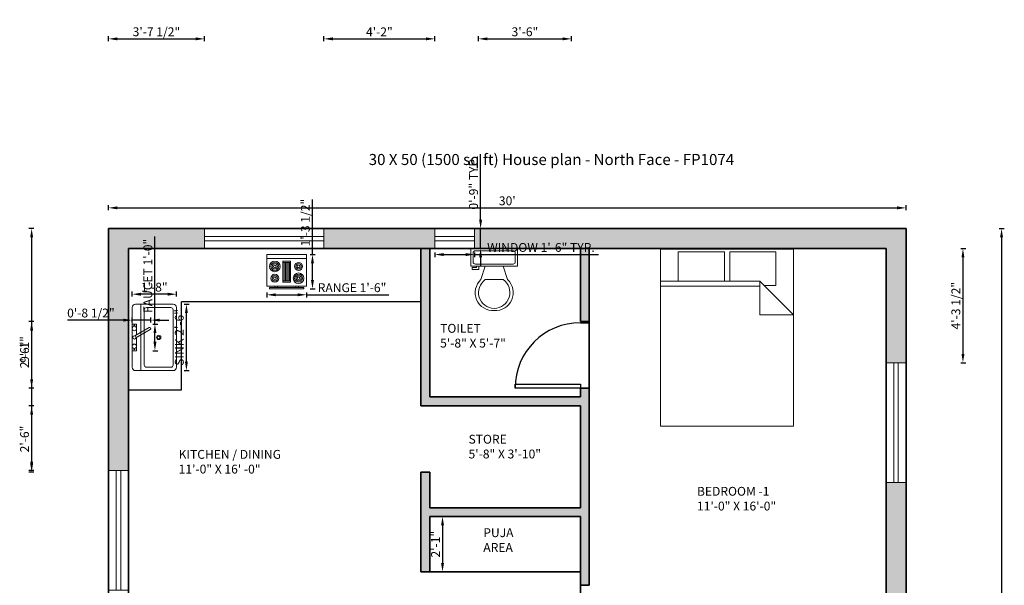
# Model space of a CAD drawing. Units: inches. Extents: x -40 to 407, y -627 to 108.
# Tile 2 of 2: x -37 to 407, y -147 to 108. Entities that reach past the tile are written whole.
import ezdxf

# ---------------------------------------------------------------- set-up
doc = ezdxf.new("R2010")
doc.units = ezdxf.units.IN
for name, color, linetype, lineweight in [('A-ANNO-DIMS', 2, 'Continuous', 18), ('A-ANNO-TEXT', 7, 'Continuous', 18), ('A-AREA-IDEN', 7, 'Continuous', 18), ('A-DOOR', 4, 'Continuous', 25), ('A-EQPM', 9, 'Continuous', 18), ('A-FLOR-CASE', 7, 'Continuous', 25), ('A-FLOR-FIXT', 8, 'Continuous', 18), ('A-FURN', 8, 'Continuous', 18), ('A-GLAZ', 6, 'Continuous', 18), ('A-WALL', 7, 'Continuous', 35), ('A-WALL-PATT', 251, 'Continuous', 13)]:
    doc.layers.add(name, color=color, linetype=linetype, lineweight=lineweight)
doc.styles.get("Standard").update_dxf_attribs({"font": 'arial.ttf'})
doc.dimstyles.new('ISO-25', dxfattribs={"dimtxt": 4, "dimasz": 4, "dimexe": 1.25, "dimexo": 0.625, "dimtad": 1, "dimlunit": 3, "dimtxsty": 'Standard', "dimcen": 2.5, "dimadec": 0, "dimazin": 0, "dimtfac": 1, "dimtmove": 0, "dimatfit": 3, "dimfxl": 1, "dimfxlon": 1, "dimarcsym": 0})

# ---------------------------------------------------------------- blocks, each defined once
blk = doc.blocks.new('*U4')
for p, q in [((0, 0), (0, -100)), ((750, 0), (750, -100))]:
    blk.add_line(p, q)
blk.add_lwpolyline([(0, 0), (0, 750), (43.75, 750), (43.75, 0)], close=True)
blk.add_arc((0, 0), 750, 0, 90)
blk = doc.blocks.new('*U2')
for p, q in [((9.5, -6), (9.5, -2)), ((-10, -8.5), (-8, -8.5)), ((-10, -9.5), (-10, -8.5)), ((-8, -8.5), (-8, -8)), ((-7, -8), (-7, -9.5)), ((-4, -8), (-6, -14)), ((4, -8), (6, -14)), ((-7, -9.5), (-10, -9.5)), ((4, -14), (-4, -14))]:
    blk.add_line(p, q)
blk.add_lwpolyline([(10.5, -8), (10.5, 0), (-10.5, 0), (-10.5, -8)], close=True)
for points in [[(-9.5, -2), (-9.5, -6)], [(8.5, -1), (-8.5, -1)], [(-8.5, -7), (8.5, -7)]]:
    blk.add_lwpolyline(points)
for centre, radius, start, end in [((-8.625, -1.875), 0.8839, 81.8699, 188.1301), ((8.625, -1.875), 0.8839, 351.8699, 98.1301), ((-8.625, -6.125), 0.8839, 171.869898, 278.1301), ((8.625, -6.125), 0.8839, 261.8699, 8.1301), ((-0.4772, -19.9188), 8.0953, 133.01722, 273.38), ((0.0374, -19.8731), 7.127, 124.50543, 269.7), ((-0.0373, -19.8731), 7.127, 270.3, 55.4946), ((0.4773, -19.9188), 8.0953, 266.62, 46.9828)]:
    blk.add_arc(centre, radius, start, end)
blk = doc.blocks.new('Sink-single - 30 in top')
blk.add_line((-15, -3.999996), (15, -3.999996))
for points in [[(-13.5, 0), (13.5, 0)], [(-15, -18.499996), (-15, -1.5)], [(15, -1.5), (15, -18.499996)], [(-13.5, -17.499996), (-13.5, -6.499996)], [(-12.5, -5.499996), (12.5, -5.499996)], [(13.5, -6.499996), (13.5, -17.499996)], [(13.5, -19.999996), (-13.5, -19.999996)], [(12.5, -18.499996), (-12.5, -18.499996)]]:
    blk.add_lwpolyline(points)
for radius in [1, 0.5]:
    blk.add_circle((0, -11.999996), radius)
for centre, radius, start, end in [((-13.5, -1.5), 1.5, 90, 180), ((13.5, -1.5), 1.5, 0, 90), ((-12.5, -6.499996), 1, 90, 180), ((12.5, -6.499996), 1, 0, 90), ((-12.5, -17.499996), 1, 180, 270), ((12.5, -17.499996), 1, 270, 0), ((-13.5, -18.499996), 1.5, 180, 270), ((13.5, -18.499996), 1.5, 270, 0)]:
    blk.add_arc(centre, radius, start, end)
blk = doc.blocks.new('Faucet - kit sink top')
for p, q in [((-5.5, -0.75), (-5.5, -1.25)), ((-4.94278, -0.75), (-5.5, -0.75)), ((-5.5, -1.25), (-4.94278, -1.25)), ((-0.14775, -1.7441), (3.56698, -8.1782)), ((4.43301, -7.6782), (0.71828, -1.2441)), ((4.94278, -0.75), (5.5, -0.75)), ((5.5, -1.25), (4.94278, -1.25)), ((5.5, -0.75), (5.5, -1.25))]:
    blk.add_line(p, q)
blk.add_lwpolyline([(-0.00587, -2), (-6, -2), (-6, 0), (6, 0), (6, -2), (1.15195, -2)])
for centre, radius in [((-4, -1), 1), ((4, -1), 1), ((0, -1), 0.75)]:
    blk.add_circle(centre, radius)
blk.add_arc((4, -7.9282), 0.5, 210, 30)
blk = doc.blocks.new('Range-Oven - 30 in top')
for p, q in [((0, -3), (30, -3)), ((12, -6), (18, -6)), ((13, -20), (13, -6)), ((14, -6), (14, -20)), ((15, -20), (15, -6)), ((16, -6), (16, -20)), ((17, -20), (17, -6)), ((18, -20), (12, -20)), ((6, -24), (6, -25)), ((8, -25), (8, -24)), ((22, -25), (22, -24)), ((24, -24), (24, -25))]:
    blk.add_line(p, q)
for points in [[(0, -24), (0, 0), (30, 0), (30, -24)], [(12, -21), (12, -5), (18, -5), (18, -21)], [(2, -26), (2, -25), (28, -25), (28, -26)]]:
    blk.add_lwpolyline(points, close=True)
for centre, radius in [((6, -9), 4), ((6, -9), 3), ((6, -9), 2), ((24, -9), 3), ((24, -9), 2), ((6, -9), 1), ((24, -18), 4), ((24, -9), 1), ((6, -18), 3), ((6, -18), 2), ((6, -18), 1), ((24, -18), 3), ((24, -18), 2), ((24, -18), 1)]:
    blk.add_circle(centre, radius)
blk = doc.blocks.new('Bed - Queen')
for p, q in [((0, -80.00003), (0, 0)), ((0, 0), (59.99999, 0)), ((59.99999, 0), (59.99999, -80.00003)), ((7.99999, -1.2), (28.79998, -1.2)), ((7.99999, -14.4), (7.99999, -1.2)), ((28.79998, -1.2), (28.79998, -14.4)), ((31.19999, -1.2), (51.99999, -1.2)), ((31.19999, -14.4), (31.19999, -1.2)), ((51.99999, -1.2), (51.99999, -16.4)), ((0, -14.4), (44.8, -14.4)), ((44.8, -16.8), (0, -16.8)), ((59.99999, -29.6), (44.8, -14.4)), ((44.8, -14.4), (44.8, -29.6)), ((51.99999, -16.4), (46.79936, -16.4)), ((44.8, -29.6), (59.99999, -29.6)), ((59.99999, -80.00003), (0, -80.00003))]:
    blk.add_line(p, q)
blk = doc.blocks.new('*D9')
at = {"layer": 'A-ANNO-DIMS', "color": 0, "lineweight": -2, "transparency": 16777216}
for p, q in [((152.9, -116.12), (155.15, -116.12)), ((153.9, -120.12), (153.9, -137.12)), ((152.9, -141.12), (155.15, -141.12))]:
    blk.add_line(p, q, dxfattribs=at)
at = {"layer": 'A-ANNO-DIMS', "color": 0, "transparency": 16777216}
for points in [[(153.23, -120.12), (154.56, -120.12), (153.9, -116.12)], [(153.23, -137.12), (154.56, -137.12), (153.9, -141.12)]]:
    blk.add_solid(points, dxfattribs=at)
at = {"layer": 'Defpoints', "color": 0, "transparency": 16777216}
for p in [(148.12, -116.12), (148.12, -141.12), (153.9, -141.12)]:
    blk.add_point(p, dxfattribs=at)
at = {"layer": 'A-ANNO-DIMS', "color": 0, "transparency": 16777216, "insert": (151.26, -128.62), "char_height": 4, "attachment_point": 5, "rotation": 90}
blk.add_mtext('2\'-1"', dxfattribs=at)
blk = doc.blocks.new('*D13')
at = {"layer": 'A-ANNO-DIMS', "color": 0, "lineweight": -2, "transparency": 16777216}
for p, q in [((3.12, 22.26), (3.12, 24.51)), ((7.12, 23.26), (359.12, 23.26)), ((363.12, 22.26), (363.12, 24.51))]:
    blk.add_line(p, q, dxfattribs=at)
at = {"layer": 'A-ANNO-DIMS', "color": 0, "transparency": 16777216}
for points in [[(7.12, 23.93), (7.12, 22.59), (3.12, 23.26)], [(359.12, 23.93), (359.12, 22.59), (363.12, 23.26)]]:
    blk.add_solid(points, dxfattribs=at)
at = {"layer": 'Defpoints', "color": 0, "transparency": 16777216}
for p in [(363.12, 23.26), (3.12, 13.88), (363.12, 13.88)]:
    blk.add_point(p, dxfattribs=at)
at = {"layer": 'A-ANNO-DIMS', "color": 0, "transparency": 16777216, "insert": (183.12, 25.93), "char_height": 4, "attachment_point": 5}
blk.add_mtext("30'", dxfattribs=at)
blk = doc.blocks.new('*D14')
at = {"layer": 'A-ANNO-DIMS', "color": 0, "lineweight": -2, "transparency": 16777216}
for p, q in [((405.24, 13.88), (407.49, 13.88)), ((406.24, 9.88), (406.24, -582.12)), ((405.24, -586.12), (407.49, -586.12))]:
    blk.add_line(p, q, dxfattribs=at)
at = {"layer": 'A-ANNO-DIMS', "color": 0, "transparency": 16777216}
for points in [[(405.57, 9.88), (406.91, 9.88), (406.24, 13.88)], [(405.57, -582.12), (406.91, -582.12), (406.24, -586.12)]]:
    blk.add_solid(points, dxfattribs=at)
at = {"layer": 'Defpoints', "color": 0, "transparency": 16777216}
for p in [(363.12, 13.88), (363.12, -586.12), (406.24, -586.12)]:
    blk.add_point(p, dxfattribs=at)
at = {"layer": 'A-ANNO-DIMS', "color": 0, "transparency": 16777216, "insert": (403.57, -286.12), "char_height": 4, "attachment_point": 5, "rotation": 90}
blk.add_mtext("50'", dxfattribs=at)
blk = doc.blocks.new('WIN-54IN')
for p, q in [((3.5, 54), (3.5, 0)), ((5.5, 54), (5.5, 0))]:
    blk.add_line(p, q)
blk.add_lwpolyline([(0, 54), (9, 54), (9, 0), (0, 0)], close=True)
blk = doc.blocks.new('WIN-18IN')
for p, q in [((18, 5.5), (0, 5.5)), ((18, 3.5), (0, 3.5))]:
    blk.add_line(p, q)
blk.add_lwpolyline([(0, 9), (18, 9), (18, 0), (0, 0)], close=True)
blk = doc.blocks.new('*D21')
at = {"layer": 'A-ANNO-DIMS', "color": 0, "lineweight": -2, "transparency": 16777216}
for p, q in [((150.38, 3.18), (150.38, 0.93)), ((154.38, 2.18), (164.38, 2.18)), ((168.38, 3.18), (168.38, 0.93)), ((168.38, 2.18), (224.25, 2.18))]:
    blk.add_line(p, q, dxfattribs=at)
at = {"layer": 'A-ANNO-DIMS', "color": 0, "transparency": 16777216}
for points in [[(154.38, 2.85), (154.38, 1.51), (150.38, 2.18)], [(164.38, 2.85), (164.38, 1.51), (168.38, 2.18)]]:
    blk.add_solid(points, dxfattribs=at)
at = {"layer": 'Defpoints', "color": 0, "transparency": 16777216}
for p in [(150.38, 4.88), (168.38, 4.88), (168.38, 2.18)]:
    blk.add_point(p, dxfattribs=at)
at = {"layer": 'A-ANNO-DIMS', "color": 0, "transparency": 16777216, "insert": (198.31, 4.87), "char_height": 4, "attachment_point": 5}
blk.add_mtext('WINDOW 1\'-6" TYP.', dxfattribs=at)
blk = doc.blocks.new('*D22')
at = {"layer": 'A-ANNO-DIMS', "color": 0, "lineweight": -2, "transparency": 16777216}
for p, q in [((171.08, 17.88), (171.08, 47.51)), ((170.08, 13.88), (172.33, 13.88)), ((171.08, 4.88), (171.08, 13.88)), ((170.08, 4.88), (172.33, 4.88)), ((171.08, 0.88), (171.08, -3.12))]:
    blk.add_line(p, q, dxfattribs=at)
at = {"layer": 'A-ANNO-DIMS', "color": 0, "transparency": 16777216}
for points in [[(170.41, 17.88), (171.75, 17.88), (171.08, 13.88)], [(170.41, 0.88), (171.75, 0.88), (171.08, 4.88)]]:
    blk.add_solid(points, dxfattribs=at)
at = {"layer": 'Defpoints', "color": 0, "transparency": 16777216}
for p in [(168.38, 13.88), (171.08, 13.88), (168.38, 4.88)]:
    blk.add_point(p, dxfattribs=at)
at = {"layer": 'A-ANNO-DIMS', "color": 0, "transparency": 16777216, "insert": (168.41, 34.7), "char_height": 4, "attachment_point": 5, "rotation": 90}
blk.add_mtext('0\'-9" TYP.', dxfattribs=at)
blk = doc.blocks.new('*D23')
at = {"layer": 'A-ANNO-DIMS', "color": 0, "lineweight": -2, "transparency": 16777216}
for p, q in [((37.28, -20.23), (39.53, -20.23)), ((38.28, -46.23), (38.28, -24.23)), ((37.28, -50.23), (39.53, -50.23))]:
    blk.add_line(p, q, dxfattribs=at)
at = {"layer": 'A-ANNO-DIMS', "color": 0, "transparency": 16777216}
for points in [[(37.62, -24.23), (38.95, -24.23), (38.28, -20.23)], [(37.62, -46.23), (38.95, -46.23), (38.28, -50.23)]]:
    blk.add_solid(points, dxfattribs=at)
at = {"layer": 'Defpoints', "color": 0, "transparency": 16777216}
for p in [(33.78, -20.23), (38.28, -20.23), (33.78, -50.23)]:
    blk.add_point(p, dxfattribs=at)
at = {"layer": 'A-ANNO-DIMS', "color": 0, "transparency": 16777216, "insert": (35.59, -35.23), "char_height": 4, "attachment_point": 5, "rotation": 90}
blk.add_mtext('SINK 2\'-6"', dxfattribs=at)
blk = doc.blocks.new('*D24')
at = {"layer": 'A-ANNO-DIMS', "color": 0, "lineweight": -2, "transparency": 16777216}
for p, q in [((13.78, -16.73), (13.78, -14.48)), ((29.78, -15.73), (17.78, -15.73)), ((33.78, -16.73), (33.78, -14.48))]:
    blk.add_line(p, q, dxfattribs=at)
at = {"layer": 'A-ANNO-DIMS', "color": 0, "transparency": 16777216}
for points in [[(17.78, -15.06), (17.78, -16.4), (13.78, -15.73)], [(29.78, -15.06), (29.78, -16.4), (33.78, -15.73)]]:
    blk.add_solid(points, dxfattribs=at)
at = {"layer": 'Defpoints', "color": 0, "transparency": 16777216}
for p in [(13.78, -15.73), (13.78, -20.23), (33.78, -20.23)]:
    blk.add_point(p, dxfattribs=at)
at = {"layer": 'A-ANNO-DIMS', "color": 0, "transparency": 16777216, "insert": (23.78, -13.06), "char_height": 4, "attachment_point": 5}
blk.add_mtext('1\'-8"', dxfattribs=at)
blk = doc.blocks.new('*D25')
at = {"layer": 'A-ANNO-DIMS', "color": 0, "lineweight": -2, "transparency": 16777216}
for p, q in [((24.08, -29.23), (24.08, 10.33)), ((23.08, -29.23), (25.33, -29.23)), ((24.08, -37.23), (24.08, -33.23)), ((23.08, -41.23), (25.33, -41.23))]:
    blk.add_line(p, q, dxfattribs=at)
at = {"layer": 'A-ANNO-DIMS', "color": 0, "transparency": 16777216}
for points in [[(23.42, -33.23), (24.75, -33.23), (24.08, -29.23)], [(23.42, -37.23), (24.75, -37.23), (24.08, -41.23)]]:
    blk.add_solid(points, dxfattribs=at)
at = {"layer": 'Defpoints', "color": 0, "transparency": 16777216}
for p in [(22.28, -29.23), (24.08, -29.23), (22.28, -41.23)]:
    blk.add_point(p, dxfattribs=at)
at = {"layer": 'A-ANNO-DIMS', "color": 0, "transparency": 16777216, "insert": (21.39, -7.45), "char_height": 4, "attachment_point": 5, "rotation": 90}
blk.add_mtext('FAUCET 1\'-0"', dxfattribs=at)
blk = doc.blocks.new('*D26')
at = {"layer": 'A-ANNO-DIMS', "color": 0, "lineweight": -2, "transparency": 16777216}
for p, q in [((13.78, -28.43), (13.78, -26.18)), ((22.28, -28.43), (22.28, -26.18)), ((9.78, -27.43), (-15.42, -27.43)), ((22.28, -27.43), (13.78, -27.43)), ((26.28, -27.43), (30.28, -27.43))]:
    blk.add_line(p, q, dxfattribs=at)
at = {"layer": 'A-ANNO-DIMS', "color": 0, "transparency": 16777216}
for points in [[(9.78, -26.76), (9.78, -28.1), (13.78, -27.43)], [(26.28, -26.76), (26.28, -28.1), (22.28, -27.43)]]:
    blk.add_solid(points, dxfattribs=at)
at = {"layer": 'Defpoints', "color": 0, "transparency": 16777216}
for p in [(13.78, -27.43), (13.78, -29.23), (22.28, -29.23)]:
    blk.add_point(p, dxfattribs=at)
at = {"layer": 'A-ANNO-DIMS', "color": 0, "transparency": 16777216, "insert": (-4.82, -24.74), "char_height": 4, "attachment_point": 5}
blk.add_mtext('0\'-8 1/2"', dxfattribs=at)
blk = doc.blocks.new('*D27')
at = {"layer": 'A-ANNO-DIMS', "color": 0, "lineweight": -2, "transparency": 16777216}
for p, q in [((74.61, -14.99), (74.61, -17.24)), ((78.61, -15.99), (88.5, -15.99)), ((92.5, -14.99), (92.5, -17.24)), ((92.5, -15.99), (129.6, -15.99))]:
    blk.add_line(p, q, dxfattribs=at)
at = {"layer": 'A-ANNO-DIMS', "color": 0, "transparency": 16777216}
for points in [[(78.61, -15.32), (78.61, -16.66), (74.61, -15.99)], [(88.5, -15.32), (88.5, -16.66), (92.5, -15.99)]]:
    blk.add_solid(points, dxfattribs=at)
at = {"layer": 'Defpoints', "color": 0, "transparency": 16777216}
for p in [(74.61, -13.31), (92.5, -13.31), (92.5, -15.99)]:
    blk.add_point(p, dxfattribs=at)
at = {"layer": 'A-ANNO-DIMS', "color": 0, "transparency": 16777216, "insert": (113.05, -13.3), "char_height": 4, "attachment_point": 5}
blk.add_mtext('RANGE 1\'-6"', dxfattribs=at)
blk = doc.blocks.new('*D28')
at = {"layer": 'A-ANNO-DIMS', "color": 0, "lineweight": -2, "transparency": 16777216}
for p, q in [((95.18, 2.2), (95.18, 27.02)), ((94.18, 2.2), (96.43, 2.2)), ((95.18, -9.31), (95.18, -1.8)), ((94.18, -13.31), (96.43, -13.31))]:
    blk.add_line(p, q, dxfattribs=at)
at = {"layer": 'A-ANNO-DIMS', "color": 0, "transparency": 16777216}
for points in [[(94.52, -1.8), (95.85, -1.8), (95.18, 2.2)], [(94.52, -9.31), (95.85, -9.31), (95.18, -13.31)]]:
    blk.add_solid(points, dxfattribs=at)
at = {"layer": 'Defpoints', "color": 0, "transparency": 16777216}
for p in [(92.5, 2.2), (95.18, 2.2), (92.5, -13.31)]:
    blk.add_point(p, dxfattribs=at)
at = {"layer": 'A-ANNO-DIMS', "color": 0, "transparency": 16777216, "insert": (92.49, 16.61), "char_height": 4, "attachment_point": 5, "rotation": 90}
blk.add_mtext('1\'-3 1/2"', dxfattribs=at)
blk = doc.blocks.new('*D29')
at = {"layer": 'A-ANNO-DIMS', "color": 0, "lineweight": -2, "transparency": 16777216}
for p, q in [((3.12, 98.58), (3.12, 100.83)), ((7.12, 99.58), (42.39, 99.58)), ((46.39, 98.58), (46.39, 100.83))]:
    blk.add_line(p, q, dxfattribs=at)
at = {"layer": 'A-ANNO-DIMS', "color": 0, "transparency": 16777216}
for points in [[(7.12, 100.25), (7.12, 98.91), (3.12, 99.58)], [(42.39, 100.25), (42.39, 98.91), (46.39, 99.58)]]:
    blk.add_solid(points, dxfattribs=at)
at = {"layer": 'Defpoints', "color": 0, "transparency": 16777216}
for p in [(46.39, 99.58), (3.12, 13.88), (46.39, 13.88)]:
    blk.add_point(p, dxfattribs=at)
at = {"layer": 'A-ANNO-DIMS', "color": 0, "transparency": 16777216, "insert": (24.75, 102.27), "char_height": 4, "attachment_point": 5}
blk.add_mtext('3\'-7 1/2"', dxfattribs=at)
blk = doc.blocks.new('*D30')
at = {"layer": 'A-ANNO-DIMS', "color": 0, "lineweight": -2, "transparency": 16777216}
for p, q in [((100.39, 98.58), (100.39, 100.83)), ((104.39, 99.58), (146.38, 99.58)), ((150.38, 98.58), (150.38, 100.83))]:
    blk.add_line(p, q, dxfattribs=at)
at = {"layer": 'A-ANNO-DIMS', "color": 0, "transparency": 16777216}
for points in [[(104.39, 100.25), (104.39, 98.91), (100.39, 99.58)], [(146.38, 100.25), (146.38, 98.91), (150.38, 99.58)]]:
    blk.add_solid(points, dxfattribs=at)
at = {"layer": 'Defpoints', "color": 0, "transparency": 16777216}
for p in [(150.38, 99.58), (100.39, 13.88), (150.38, 13.88)]:
    blk.add_point(p, dxfattribs=at)
at = {"layer": 'A-ANNO-DIMS', "color": 0, "transparency": 16777216, "insert": (125.39, 102.21), "char_height": 4, "attachment_point": 5}
blk.add_mtext('4\'-2"', dxfattribs=at)
blk = doc.blocks.new('*D31')
at = {"layer": 'A-ANNO-DIMS', "color": 0, "lineweight": -2, "transparency": 16777216}
for p, q in [((-30.58, -66.12), (-32.83, -66.12)), ((-31.58, -70.12), (-31.58, -92.12)), ((-30.58, -96.12), (-32.83, -96.12))]:
    blk.add_line(p, q, dxfattribs=at)
at = {"layer": 'A-ANNO-DIMS', "color": 0, "transparency": 16777216}
for points in [[(-32.25, -70.12), (-30.91, -70.12), (-31.58, -66.12)], [(-32.25, -92.12), (-30.91, -92.12), (-31.58, -96.12)]]:
    blk.add_solid(points, dxfattribs=at)
at = {"layer": 'Defpoints', "color": 0, "transparency": 16777216}
for p in [(144.12, -66.12), (-31.58, -96.12), (144.12, -96.12)]:
    blk.add_point(p, dxfattribs=at)
at = {"layer": 'A-ANNO-DIMS', "color": 0, "transparency": 16777216, "insert": (-34.25, -81.12), "char_height": 4, "attachment_point": 5, "rotation": 90}
blk.add_mtext('2\'-6"', dxfattribs=at)
blk = doc.blocks.new('*D32')
at = {"layer": 'A-ANNO-DIMS', "color": 0, "lineweight": -2, "transparency": 16777216}
for p, q in [((-30.58, -28.12), (-32.83, -28.12)), ((-31.58, -32.12), (-31.58, -54.12)), ((-30.58, -58.12), (-32.83, -58.12))]:
    blk.add_line(p, q, dxfattribs=at)
at = {"layer": 'A-ANNO-DIMS', "color": 0, "transparency": 16777216}
for points in [[(-32.25, -32.12), (-30.91, -32.12), (-31.58, -28.12)], [(-32.25, -54.12), (-30.91, -54.12), (-31.58, -58.12)]]:
    blk.add_solid(points, dxfattribs=at)
at = {"layer": 'Defpoints', "color": 0, "transparency": 16777216}
for p in [(216.12, -28.12), (-31.58, -58.12), (216.12, -58.12)]:
    blk.add_point(p, dxfattribs=at)
at = {"layer": 'A-ANNO-DIMS', "color": 0, "transparency": 16777216, "insert": (-34.25, -43.12), "char_height": 4, "attachment_point": 5, "rotation": 90}
blk.add_mtext('2\'-6"', dxfattribs=at)
blk = doc.blocks.new('*D34')
at = {"layer": 'A-ANNO-DIMS', "color": 0, "lineweight": -2, "transparency": 16777216}
for p, q in [((170.1, 98.58), (170.1, 100.83)), ((174.1, 99.58), (208.1, 99.58)), ((212.1, 98.58), (212.1, 100.83))]:
    blk.add_line(p, q, dxfattribs=at)
at = {"layer": 'A-ANNO-DIMS', "color": 0, "transparency": 16777216}
for points in [[(174.1, 100.25), (174.1, 98.91), (170.1, 99.58)], [(208.1, 100.25), (208.1, 98.91), (212.1, 99.58)]]:
    blk.add_solid(points, dxfattribs=at)
at = {"layer": 'Defpoints', "color": 0, "transparency": 16777216}
for p in [(212.1, 99.58), (170.1, -443.12), (212.1, -443.12)]:
    blk.add_point(p, dxfattribs=at)
at = {"layer": 'A-ANNO-DIMS', "color": 0, "transparency": 16777216, "insert": (191.1, 102.25), "char_height": 4, "attachment_point": 5}
blk.add_mtext('3\'-6"', dxfattribs=at)
blk = doc.blocks.new('*D35')
at = {"layer": 'A-ANNO-DIMS', "color": 0, "lineweight": -2, "transparency": 16777216}
for p, q in [((-30.58, 13.88), (-32.83, 13.88)), ((-31.58, 9.88), (-31.58, -91.31)), ((-30.58, -95.31), (-32.83, -95.31))]:
    blk.add_line(p, q, dxfattribs=at)
at = {"layer": 'A-ANNO-DIMS', "color": 0, "transparency": 16777216}
for points in [[(-32.25, 9.88), (-30.91, 9.88), (-31.58, 13.88)], [(-32.25, -91.31), (-30.91, -91.31), (-31.58, -95.31)]]:
    blk.add_solid(points, dxfattribs=at)
at = {"layer": 'Defpoints', "color": 0, "transparency": 16777216}
for p in [(3.12, 13.88), (-31.58, -95.31), (3.12, -95.31)]:
    blk.add_point(p, dxfattribs=at)
at = {"layer": 'A-ANNO-DIMS', "color": 0, "transparency": 16777216, "insert": (-34.25, -40.71), "char_height": 4, "attachment_point": 5, "rotation": 90}
blk.add_mtext('9\'-1"', dxfattribs=at)
blk = doc.blocks.new('*D38')
at = {"layer": 'A-ANNO-DIMS', "color": 0, "lineweight": -2, "transparency": 16777216}
for p, q in [((387.82, 4.88), (390.07, 4.88)), ((388.82, 0.88), (388.82, -42.69)), ((387.82, -46.69), (390.07, -46.69))]:
    blk.add_line(p, q, dxfattribs=at)
at = {"layer": 'A-ANNO-DIMS', "color": 0, "transparency": 16777216}
for points in [[(388.15, 0.88), (389.49, 0.88), (388.82, 4.88)], [(388.15, -42.69), (389.49, -42.69), (388.82, -46.69)]]:
    blk.add_solid(points, dxfattribs=at)
at = {"layer": 'Defpoints', "color": 0, "transparency": 16777216}
for p in [(354.12, 4.88), (354.12, -46.69), (388.82, -46.69)]:
    blk.add_point(p, dxfattribs=at)
at = {"layer": 'A-ANNO-DIMS', "color": 0, "transparency": 16777216, "insert": (386.13, -20.91), "char_height": 4, "attachment_point": 5, "rotation": 90}
blk.add_mtext('4\'-3 1/2"', dxfattribs=at)

msp = doc.modelspace()

# ---------------------------------------------------------------- hatches: boundary and pattern name
at = {"layer": 'A-WALL-PATT'}
h = msp.add_hatch(color=256, dxfattribs=at)
h.dxf.hatch_style = 1
h.paths.add_polyline_path([(12.12, 4.879), (46.39, 4.879), (46.39, 13.879), (3.12, 13.879), (3.12, -95.306), (12.12, -95.306)])
h.paths.add_polyline_path([(150.38, 13.879), (100.39, 13.879), (100.39, 4.879), (144.12, 4.879), (148.12, 4.879), (150.38, 4.879)])
h.paths.add_polyline_path([(363.12, 13.879), (168.38, 13.879), (168.38, 4.879), (187.717, 4.879), (216.12, 4.879), (220.12, 4.879), (354.12, 4.879), (354.12, -46.69), (363.12, -46.69)])
h.paths.add_polyline_path([(148.12, 4.879), (144.12, 4.879), (144.12, -66.121), (148.12, -66.121), (216.12, -66.121), (216.12, -112.121), (148.12, -112.121), (148.12, -96.121), (144.12, -96.121), (144.12, -141.121), (148.12, -141.121), (148.12, -116.121), (216.12, -116.121), (216.12, -147.121), (220.12, -147.121), (220.12, -58.121), (216.12, -58.121), (216.12, -62.121), (148.12, -62.121)])
h.paths.add_polyline_path([(220.12, 4.879), (216.12, 4.879), (216.12, -28.121), (220.12, -28.121)], flags=17)
h.paths.add_polyline_path([(363.12, -100.69), (354.12, -100.69), (354.12, -236.329), (363.12, -236.329)])
h.paths.add_polyline_path([(354.12, -187.121), (220.12, -187.121), (220.12, -183.121), (216.12, -183.121), (216.12, -271.121), (220.12, -271.121), (220.12, -191.121), (354.12, -191.121)])
h.paths.add_polyline_path([(363.12, -441.809), (354.12, -441.809), (354.12, -577.121), (330.838, -577.121), (330.838, -586.121), (363.12, -586.121)])
h.paths.add_polyline_path([(363.12, -372.174), (354.12, -372.174), (354.12, -391.121), (354.12, -423.809), (363.12, -423.809)])
h.paths.add_polyline_path([(354.12, -443.121), (270.12, -443.121), (270.12, -429.121), (266.12, -429.121), (266.12, -443.121), (260.12, -443.121), (260.12, -447.121), (266.12, -447.121), (270.12, -447.121), (354.12, -447.121)])
h.paths.add_polyline_path([(354.12, -391.121), (216.12, -391.121), (216.12, -395.121), (266.12, -395.121), (266.12, -399.121), (270.12, -399.121), (270.12, -395.121), (354.12, -395.121)])
h.paths.add_polyline_path([(354.12, -311.121), (220.12, -311.121), (220.12, -307.121), (216.12, -307.121), (216.12, -315.121), (354.12, -315.121)])
h.paths.add_polyline_path([(170.105, -443.121), (12.12, -443.121), (12.12, -447.121), (170.105, -447.121)])
h.paths.add_polyline_path([(12.12, -403.805), (3.12, -403.805), (3.12, -586.121), (12.12, -586.121)])
h.paths.add_polyline_path([(220.12, -447.121), (224.12, -447.121), (224.12, -443.121), (220.12, -443.121), (216.12, -443.121), (212.105, -443.121), (212.105, -447.121), (216.12, -447.121), (216.12, -577.121), (220.12, -577.121)])
h.paths.add_polyline_path([(276.838, -577.121), (212.099, -577.121), (212.099, -586.121), (276.838, -586.121)])

# ---------------------------------------------------------------- linework, layer by layer
at = {"layer": 'A-FLOR-CASE'}
for p, q in [((144.12, -19.121), (36.12, -19.121)), ((36.12, -58.939), (36.12, -19.121)), ((12.12, -58.939), (36.12, -58.939))]:
    msp.add_line(p, q, dxfattribs=at)
at = {"layer": 'A-WALL'}
for p, q in [((3.12, 13.879), (363.12, 13.879)), ((3.12, -586.121), (3.12, 13.879)), ((363.12, 13.879), (363.12, -586.121)), ((12.12, 4.879), (144.12, 4.879)), ((12.12, -586.121), (12.12, 4.879)), ((144.12, 4.879), (148.12, 4.879)), ((144.12, -66.121), (144.12, 4.879)), ((148.12, 4.879), (216.12, 4.879)), ((148.12, -62.121), (148.12, 4.879)), ((216.12, 4.879), (220.12, 4.879)), ((216.12, -28.121), (216.12, 4.879)), ((220.12, 4.879), (354.12, 4.879)), ((220.12, -147.121), (220.12, 4.879)), ((354.12, 4.879), (354.12, -315.121)), ((216.12, -28.121), (220.12, -28.121)), ((148.12, -62.121), (216.12, -62.121)), ((216.12, -62.121), (216.12, -58.121)), ((216.12, -58.121), (220.12, -58.121)), ((148.12, -66.121), (144.12, -66.121)), ((148.12, -66.121), (216.12, -66.121)), ((216.12, -112.121), (216.12, -66.121)), ((148.12, -96.121), (144.12, -96.121)), ((144.12, -141.121), (144.12, -96.121)), ((148.12, -112.121), (148.12, -96.121)), ((148.12, -112.121), (216.12, -112.121)), ((148.12, -116.121), (216.12, -116.121)), ((148.12, -141.121), (148.12, -116.121)), ((216.12, -315.121), (216.12, -116.121)), ((144.12, -141.121), (216.12, -141.121)), ((220.12, -147.121), (216.12, -147.121))]:
    msp.add_line(p, q, dxfattribs=at)

# ---------------------------------------------------------------- block references
at = {"layer": 'A-DOOR', "xscale": 0.0393700787401575, "yscale": 0.0393700787401575, "zscale": 0.0393700787401575, "rotation": 90}
msp.add_blockref('*U4', (216.183, -58.121), dxfattribs=at)
at = {"layer": 'A-EQPM', "xscale": 0.5962845554860383, "yscale": 0.5962845554860383, "zscale": 0.5962845554860383}
msp.add_blockref('Range-Oven - 30 in top', (74.611, 2.198), dxfattribs=at)
at = {"layer": 'A-FLOR-FIXT'}
msp.add_blockref('*U2', (177.217, 4.879), dxfattribs=at)
at = {"layer": 'A-FLOR-FIXT', "rotation": 90}
for name in ['Sink-single - 30 in top', 'Faucet - kit sink top']:
    msp.add_blockref(name, (13.783, -35.229), dxfattribs=at)
at = {"layer": 'A-FURN'}
msp.add_blockref('Bed - Queen', (252.331, 4.631), dxfattribs=at)
at = {"layer": 'A-GLAZ', "rotation": 270}
msp.add_blockref('WIN-54IN', (46.389, 13.879), dxfattribs=at)
at = {"layer": 'A-GLAZ'}
for name, p in [('WIN-18IN', (150.38, 4.879)), ('WIN-54IN', (354.12, -100.69)), ('WIN-54IN', (3.12, -149.306))]:
    msp.add_blockref(name, p, dxfattribs=at)

# ---------------------------------------------------------------- texts
at = {"layer": 'A-ANNO-TEXT', "insert": (120.574, 47.603), "char_height": 5, "attachment_point": 1}
msp.add_mtext_dynamic_manual_height_columns('30 X 50 (1500 sq ft) House plan - North Face - FP1074', width=380.28453, gutter_width=12.5, heights=[0], dxfattribs=at)
at = {"layer": 'A-AREA-IDEN', "char_height": 4, "attachment_point": 1}
for s, width, insert in [('TOILET\\P5\'-8" X 5\'-7"', 39.09171, (152.822, -29.137)), ('STORE\\P5\'-8" X 3\'-10"', 41.51332, (165.642, -79.212)), ('KITCHEN / DINING\\P11\'-0" X 16\' -0"', 81.1131, (34.792, -86.045)), ('BEDROOM -1\\P11\'-0" X 16\'-0"', 89.67245, (268.764, -102.729)), ('PUJA\\PAREA', 32.98523, (172.305, -121.419))]:
    msp.add_mtext_dynamic_manual_height_columns(s, width=width, gutter_width=12.5, heights=[0], dxfattribs=dict(at, insert=insert))

# ---------------------------------------------------------------- dimensions: what is measured, and where the dimension line sits
at = {"layer": 'A-ANNO-DIMS'}
for base, p1, p2, override, picture, middle in [((46.39, 99.579), (3.12, 13.879), (46.39, 13.879), {"dimdec": 1, "dimlfac": 1, "dimrnd": 0, "dimzin": 1, "dimdsep": 46, "dimlunit": 4, "dimfrac": 2}, '*D29', (24.755, 102.274)), ((150.38, 99.579), (100.39, 13.879), (150.38, 13.879), {"dimdec": 1, "dimlfac": 1, "dimrnd": 0, "dimzin": 1, "dimdsep": 46, "dimlunit": 4, "dimfrac": 2}, '*D30', (125.385, 102.212)), ((212.105, 99.579), (170.105, -443.121), (212.105, -443.121), {"dimdec": 1, "dimlfac": 1, "dimrnd": 0, "dimzin": 1, "dimdsep": 46, "dimlunit": 4, "dimfrac": 2}, '*D34', (191.105, 102.248)), ((363.12, 23.26), (3.12, 13.879), (363.12, 13.879), {"dimclrd": 0, "dimclre": 0, "dimclrt": 0}, '*D13', (183.12, 25.929))]:
    dim = msp.add_linear_dim(base=base, p1=p1, p2=p2, dimstyle='ISO-25', override=override, dxfattribs=at)
    dim.commit()
    dim.dimension.update_dxf_attribs({"geometry": picture, "text_midpoint": middle})
for base, p1, p2, text, picture, middle in [((171.08, 13.879), (168.38, 4.879), (168.38, 13.879), '<> TYP.', '*D22', (168.413, 34.695)), ((24.082, -29.229), (22.282, -41.229), (22.282, -29.229), 'FAUCET <>', '*D25', (21.389, -7.449)), ((38.283, -20.229), (33.783, -50.229), (33.783, -20.229), 'SINK <>', '*D23', (35.59, -35.229))]:
    dim = msp.add_linear_dim(base=base, p1=p1, p2=p2, angle=90, text=text, dimstyle='ISO-25', override={"dimdec": 1, "dimlfac": 1, "dimrnd": 0, "dimzin": 1, "dimdsep": 46, "dimlunit": 4, "dimfrac": 2}, dxfattribs=at)
    dim.commit()
    dim.dimension.update_dxf_attribs({"geometry": picture, "text_midpoint": middle})
for base, p1, p2, angle, override, picture, middle in [((95.183, 2.198), (92.5, -13.306), (92.5, 2.198), 90, {"dimdec": 1, "dimlfac": 1, "dimrnd": 0, "dimzin": 1, "dimdsep": 46, "dimlunit": 4, "dimfrac": 2}, '*D28', (92.489, 16.611)), ((-31.58, -95.306), (3.12, 13.879), (3.12, -95.306), 90, {"dimdec": 1, "dimlfac": 1, "dimrnd": 0, "dimzin": 1, "dimdsep": 46, "dimlunit": 4, "dimfrac": 2}, '*D35', (-34.248, -40.713)), ((406.24, -586.121), (363.12, 13.879), (363.12, -586.121), 90, {"dimclrd": 0, "dimclre": 0, "dimclrt": 0}, '*D14', (403.573, -286.121)), ((388.82, -46.69), (354.12, 4.879), (354.12, -46.69), 270, {"dimdec": 1, "dimlfac": 1, "dimrnd": 0, "dimzin": 1, "dimdsep": 46, "dimlunit": 4, "dimfrac": 2}, '*D38', (386.125, -20.905)), ((13.783, -15.729), (33.783, -20.229), (13.783, -20.229), 180, {"dimdec": 1, "dimlfac": 1, "dimrnd": 0, "dimzin": 1, "dimdsep": 46, "dimlunit": 4, "dimfrac": 2}, '*D24', (23.783, -13.062)), ((13.783, -27.429), (22.282, -29.229), (13.783, -29.229), 180, {"dimdec": 1, "dimlfac": 1, "dimrnd": 0, "dimzin": 1, "dimdsep": 46, "dimlunit": 4, "dimfrac": 2}, '*D26', (-4.819, -24.736)), ((-31.58, -58.121), (216.12, -28.121), (216.12, -58.121), 90, {"dimdec": 1, "dimlfac": 1, "dimrnd": 0, "dimzin": 1, "dimdsep": 46, "dimlunit": 4, "dimfrac": 2}, '*D32', (-34.248, -43.121)), ((-31.58, -96.121), (144.12, -66.121), (144.12, -96.121), 90, {"dimdec": 1, "dimlfac": 1, "dimrnd": 0, "dimzin": 1, "dimdsep": 46, "dimlunit": 4, "dimfrac": 2}, '*D31', (-34.248, -81.121)), ((153.897, -141.121), (148.12, -116.121), (148.12, -141.121), 90, {"dimclrd": 0, "dimclre": 0, "dimclrt": 0}, '*D9', (151.263, -128.621))]:
    dim = msp.add_linear_dim(base=base, p1=p1, p2=p2, angle=angle, dimstyle='ISO-25', override=override, dxfattribs=at)
    dim.commit()
    dim.dimension.update_dxf_attribs({"geometry": picture, "text_midpoint": middle})
for base, p1, p2, text, picture, middle in [((168.38, 2.179), (150.38, 4.879), (168.38, 4.879), 'WINDOW <> TYP.', '*D21', (198.314, 4.874)), ((92.5, -15.989), (74.611, -13.306), (92.5, -13.306), 'RANGE <>', '*D27', (113.05, -13.296))]:
    dim = msp.add_linear_dim(base=base, p1=p1, p2=p2, text=text, dimstyle='ISO-25', override={"dimdec": 1, "dimlfac": 1, "dimrnd": 0, "dimzin": 1, "dimdsep": 46, "dimlunit": 4, "dimfrac": 2}, dxfattribs=at)
    dim.commit()
    dim.dimension.update_dxf_attribs({"geometry": picture, "text_midpoint": middle})

doc.saveas('drawing.dxf')
